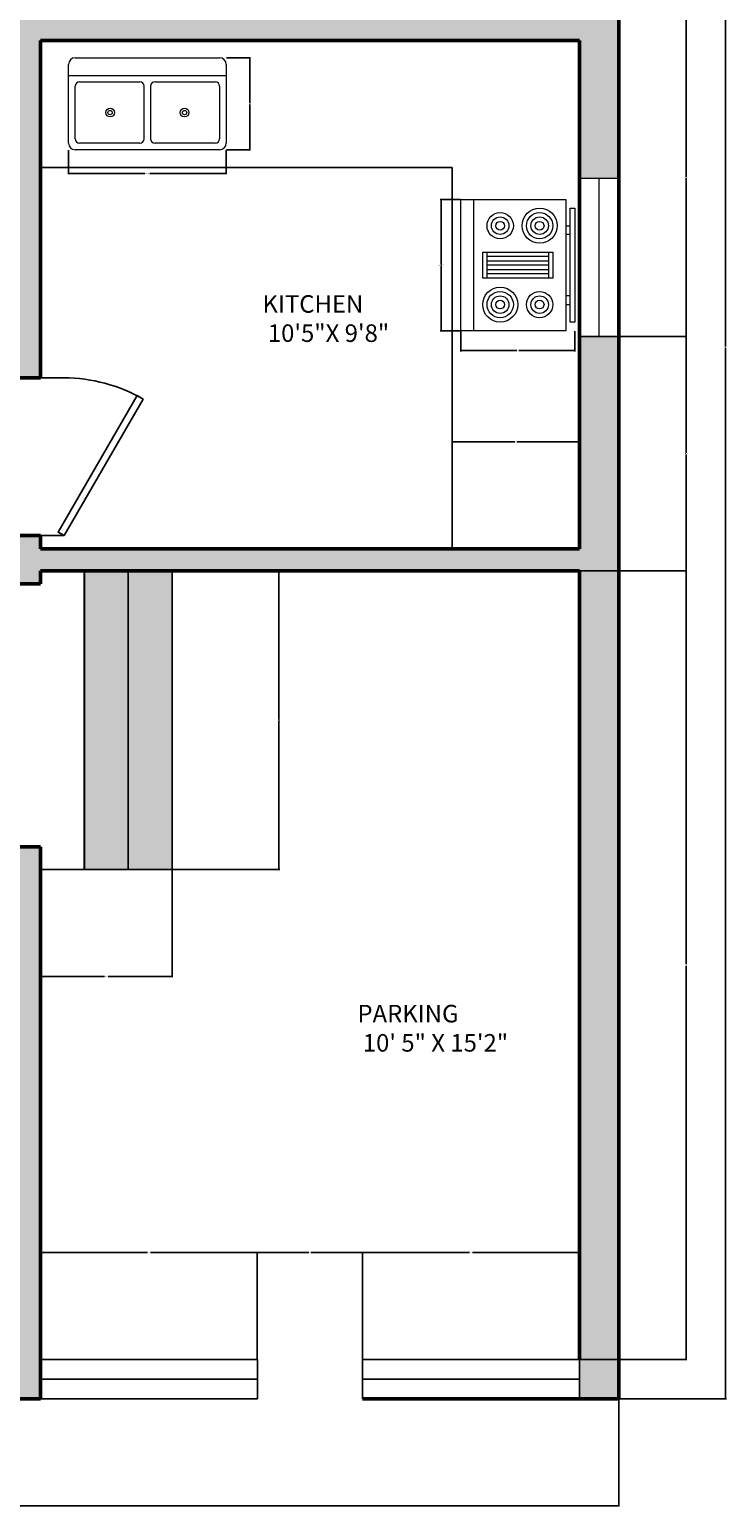
# Model space of a CAD drawing. Units: inches. Extents: x -23 to 411, y -22 to 507.
# Tile 3 of 5: x 252 to 411, y -22 to 315. Entities that reach past the tile are written whole.
import ezdxf

# ---------------------------------------------------------------- set-up
doc = ezdxf.new("R2010")
doc.units = ezdxf.units.IN
doc.header["$MEASUREMENT"] = 0
for name, color, linetype, lineweight in [('A-ANNO-DIMS', 2, 'Continuous', 18), ('A-AREA-IDEN', 7, 'Continuous', 25), ('A-EQPM', 181, 'Continuous', 18), ('A-FLOR-CASE', 181, 'Continuous', 25), ('A-FLOR-FIXT', 90, 'Continuous', 18), ('A-FLOR-STRS', 7, 'Continuous', 25), ('A-WALL', 7, 'Continuous', 50), ('doors', 40, 'Continuous', 25), ('window', 30, 'Continuous', 18)]:
    doc.layers.add(name, color=color, linetype=linetype, lineweight=lineweight)
doc.layers.add('A-FLOR-PATT', color=51, linetype='Continuous', lineweight=13, true_color=0xf8f6b0)
doc.layers.add('A-WALL-PATT', color=179, linetype='Continuous', lineweight=13, true_color=0x161b4b)
doc.styles.get("Standard").update_dxf_attribs({"font": 'arial.ttf'})
doc.dimstyles.get("Standard").update_dxf_attribs({"dimtxt": 0.18, "dimasz": 0.18, "dimexe": 0.18, "dimexo": 0.0625, "dimgap": 0.09, "dimtad": 0, "dimtih": 1, "dimtoh": 1, "dimdec": 4, "dimzin": 0, "dimdsep": 46, "dimtxsty": 'Standard', "dimcen": 0.09, "dimadec": 0, "dimazin": 0, "dimtfac": 1, "dimtdec": 4, "dimtofl": 0, "dimtmove": 0, "dimatfit": 3, "dimfxl": 1, "dimtolj": 1, "dimtzin": 0, "dimarcsym": 0})

# ---------------------------------------------------------------- blocks, each defined once
blk = doc.blocks.new('*U7')
for p, q in [((0, 0), (0, 6)), ((40, 0), (40, 6))]:
    blk.add_line(p, q)
blk.add_lwpolyline([(0, 0), (34.64, -20), (35.52, -18.48), (0.87, 1.52)], close=True)
blk.add_arc((0, 0), 40, 330, 0)
blk = doc.blocks.new('Range-Oven - 30 in top')
for p, q in [((0, -3), (30, -3)), ((12, -6), (18, -6)), ((13, -20), (13, -6)), ((14, -6), (14, -20)), ((15, -20), (15, -6)), ((16, -6), (16, -20)), ((17, -20), (17, -6)), ((18, -20), (12, -20)), ((6, -24), (6, -25)), ((8, -25), (8, -24)), ((22, -25), (22, -24)), ((24, -24), (24, -25))]:
    blk.add_line(p, q)
for points in [[(0, -24), (0, 0), (30, 0), (30, -24)], [(12, -21), (12, -5), (18, -5), (18, -21)], [(2, -26), (2, -25), (28, -25), (28, -26)]]:
    blk.add_lwpolyline(points, close=True)
for centre, radius in [((6, -9), 4), ((6, -9), 3), ((24, -9), 3), ((6, -9), 2), ((6, -9), 1), ((24, -9), 2), ((24, -9), 1), ((6, -18), 3), ((6, -18), 2), ((24, -18), 4), ((24, -18), 3), ((24, -18), 2), ((6, -18), 1), ((24, -18), 1)]:
    blk.add_circle(centre, radius)
blk = doc.blocks.new('Sink-double - 36 in top')
for p, q in [((-18, -4), (18, -4)), ((-0.75, -18.5), (-0.75, -6.5)), ((0.75, -6.5), (0.75, -18.5))]:
    blk.add_line(p, q)
for points in [[(-16.5, 0), (16.5, 0)], [(-18, -19.5), (-18, -1.5)], [(18, -1.5), (18, -19.5)], [(-16.5, -18.5), (-16.5, -6.5)], [(-15.5, -5.5), (-1.75, -5.5)], [(1.75, -5.5), (15.5, -5.5)], [(16.5, -6.5), (16.5, -18.5)], [(-1.75, -19.5), (-15.5, -19.5)], [(15.5, -19.5), (1.75, -19.5)], [(16.5, -21), (-16.5, -21)]]:
    blk.add_lwpolyline(points)
for centre, radius in [((-8.5, -12.5), 1), ((-8.5, -12.5), 0.5), ((8.5, -12.5), 1), ((8.5, -12.5), 0.5)]:
    blk.add_circle(centre, radius)
for centre, radius, start, end in [((-16.5, -1.5), 1.5, 90, 180), ((16.5, -1.5), 1.5, 0, 90), ((-15.5, -6.5), 1, 90, 180), ((-1.75, -6.5), 1, 0, 90), ((1.75, -6.5), 1, 90, 180), ((15.5, -6.5), 1, 0, 90), ((-16.5, -19.5), 1.5, 180, 270), ((-15.5, -18.5), 1, 180, 270), ((-1.75, -18.5), 1, 270, 0), ((1.75, -18.5), 1, 180, 270), ((15.5, -18.5), 1, 270, 0), ((16.5, -19.5), 1.5, 270, 0)]:
    blk.add_arc(centre, radius, start, end)
blk = doc.blocks.new('WIN-36IN')
for p, q in [((9, 36), (0, 36)), ((0, 36), (0, 0)), ((4.5, 0), (4.5, 36)), ((9, 0), (9, 36)), ((0, 0), (9, 0)), ((0, 0), (4.5, 0))]:
    blk.add_line(p, q)
blk = doc.blocks.new('*D22')
at = {"layer": 'A-ANNO-DIMS', "color": 0, "lineweight": -2, "transparency": 16777216}
for p, q in [((350.04, 276.62), (345.43, 276.62)), ((345.61, 276.44), (345.61, 261.81)), ((345.61, 246.8), (345.61, 261.44)), ((350.04, 246.62), (345.43, 246.62))]:
    blk.add_line(p, q, dxfattribs=at)
at = {"layer": 'A-ANNO-DIMS', "color": 0, "transparency": 16777216}
for points in [[(345.58, 276.44), (345.64, 276.44), (345.61, 276.62)], [(345.58, 246.8), (345.64, 246.8), (345.61, 246.62)]]:
    blk.add_solid(points, dxfattribs=at)
at = {"layer": 'Defpoints', "color": 0, "transparency": 16777216}
for p in [(345.61, 276.62), (350.11, 276.62), (350.11, 246.62)]:
    blk.add_point(p, dxfattribs=at)
at = {"layer": 'A-ANNO-DIMS', "color": 0, "transparency": 16777216, "insert": (345.61, 261.62), "char_height": 0.18, "attachment_point": 5}
blk.add_mtext('\\A1;RANGE 30', dxfattribs=at)
blk = doc.blocks.new('*D23')
at = {"layer": 'A-ANNO-DIMS', "color": 0, "lineweight": -2, "transparency": 16777216}
for p, q in [((350.11, 246.56), (350.11, 241.94)), ((376.11, 246.56), (376.11, 241.94)), ((350.29, 242.12), (362.89, 242.12)), ((375.93, 242.12), (363.33, 242.12))]:
    blk.add_line(p, q, dxfattribs=at)
at = {"layer": 'A-ANNO-DIMS', "color": 0, "transparency": 16777216}
for points in [[(350.29, 242.15), (350.29, 242.09), (350.11, 242.12)], [(375.93, 242.15), (375.93, 242.09), (376.11, 242.12)]]:
    blk.add_solid(points, dxfattribs=at)
at = {"layer": 'Defpoints', "color": 0, "transparency": 16777216}
for p in [(350.11, 246.62), (376.11, 246.62), (350.11, 242.12)]:
    blk.add_point(p, dxfattribs=at)
at = {"layer": 'A-ANNO-DIMS', "color": 0, "transparency": 16777216, "insert": (363.11, 242.12), "char_height": 0.18, "attachment_point": 5}
blk.add_mtext('\\A1;26', dxfattribs=at)
blk = doc.blocks.new('*D24')
at = {"layer": 'A-ANNO-DIMS', "color": 0, "lineweight": -2, "transparency": 16777216}
for p, q in [((260.57, 287.88), (260.57, 282.37)), ((296.57, 287.88), (296.57, 282.37)), ((260.75, 282.55), (278.02, 282.55)), ((296.39, 282.55), (279.12, 282.55))]:
    blk.add_line(p, q, dxfattribs=at)
at = {"layer": 'A-ANNO-DIMS', "color": 0, "transparency": 16777216}
for points in [[(260.75, 282.58), (260.75, 282.52), (260.57, 282.55)], [(296.39, 282.58), (296.39, 282.52), (296.57, 282.55)]]:
    blk.add_solid(points, dxfattribs=at)
at = {"layer": 'Defpoints', "color": 0, "transparency": 16777216}
for p in [(260.57, 287.95), (296.57, 287.95), (296.57, 282.55)]:
    blk.add_point(p, dxfattribs=at)
at = {"layer": 'A-ANNO-DIMS', "color": 0, "transparency": 16777216, "insert": (278.57, 282.55), "char_height": 0.18, "attachment_point": 5}
blk.add_mtext('\\A1;SINK 36', dxfattribs=at)
blk = doc.blocks.new('*D25')
at = {"layer": 'A-ANNO-DIMS', "color": 0, "lineweight": -2, "transparency": 16777216}
for p, q in [((296.63, 308.95), (302.15, 308.95)), ((301.97, 308.77), (301.97, 298.63)), ((301.97, 288.13), (301.97, 298.26)), ((296.63, 287.95), (302.15, 287.95))]:
    blk.add_line(p, q, dxfattribs=at)
at = {"layer": 'A-ANNO-DIMS', "color": 0, "transparency": 16777216}
for points in [[(301.94, 308.77), (302, 308.77), (301.97, 308.95)], [(301.94, 288.13), (302, 288.13), (301.97, 287.95)]]:
    blk.add_solid(points, dxfattribs=at)
at = {"layer": 'Defpoints', "color": 0, "transparency": 16777216}
for p in [(296.57, 308.95), (301.97, 308.95), (296.57, 287.95)]:
    blk.add_point(p, dxfattribs=at)
at = {"layer": 'A-ANNO-DIMS', "color": 0, "transparency": 16777216, "insert": (301.97, 298.45), "char_height": 0.18, "attachment_point": 5}
blk.add_mtext('\\A1;21', dxfattribs=at)
blk = doc.blocks.new('*D28')
at = {"layer": 'A-ANNO-DIMS', "color": 0, "lineweight": -2, "transparency": 16777216}
for p, q in [((2.17, 2.83), (2.17, -21.66)), ((386.17, 2.83), (386.17, -21.66)), ((2.35, -21.48), (193.89, -21.48)), ((385.99, -21.48), (194.46, -21.48))]:
    blk.add_line(p, q, dxfattribs=at)
at = {"layer": 'A-ANNO-DIMS', "color": 0, "transparency": 16777216}
for points in [[(2.35, -21.45), (2.35, -21.51), (2.17, -21.48)], [(385.99, -21.45), (385.99, -21.51), (386.17, -21.48)]]:
    blk.add_solid(points, dxfattribs=at)
at = {"layer": 'Defpoints', "color": 0, "transparency": 16777216}
for p in [(2.17, 2.9), (386.17, 2.9), (386.17, -21.48)]:
    blk.add_point(p, dxfattribs=at)
at = {"layer": 'A-ANNO-DIMS', "color": 0, "transparency": 16777216, "insert": (194.17, -21.48), "char_height": 0.18, "attachment_point": 5}
blk.add_mtext('\\A1;384', dxfattribs=at)
blk = doc.blocks.new('*D29')
at = {"layer": 'A-ANNO-DIMS', "color": 0, "lineweight": -2, "transparency": 16777216}
for p, q in [((386.24, 482.9), (410.73, 482.9)), ((410.55, 482.72), (410.55, 243.08)), ((410.55, 3.08), (410.55, 242.72)), ((386.24, 2.9), (410.73, 2.9))]:
    blk.add_line(p, q, dxfattribs=at)
at = {"layer": 'A-ANNO-DIMS', "color": 0, "transparency": 16777216}
for points in [[(410.52, 482.72), (410.58, 482.72), (410.55, 482.9)], [(410.52, 3.08), (410.58, 3.08), (410.55, 2.9)]]:
    blk.add_solid(points, dxfattribs=at)
at = {"layer": 'Defpoints', "color": 0, "transparency": 16777216}
for p in [(386.17, 482.9), (386.17, 2.9), (410.55, 2.9)]:
    blk.add_point(p, dxfattribs=at)
at = {"layer": 'A-ANNO-DIMS', "color": 0, "transparency": 16777216, "insert": (410.55, 242.9), "char_height": 0.18, "attachment_point": 5}
blk.add_mtext('\\A1;480', dxfattribs=at)
blk = doc.blocks.new('*D53')
at = {"layer": 'A-ANNO-DIMS', "color": 0, "lineweight": -2, "transparency": 16777216}
for p, q in [((377.24, 191.9), (401.73, 191.9)), ((401.55, 191.72), (401.55, 102.08)), ((401.55, 12.08), (401.55, 101.72)), ((377.24, 11.9), (401.73, 11.9))]:
    blk.add_line(p, q, dxfattribs=at)
at = {"layer": 'A-ANNO-DIMS', "color": 0, "transparency": 16777216}
for points in [[(401.52, 191.72), (401.58, 191.72), (401.55, 191.9)], [(401.52, 12.08), (401.58, 12.08), (401.55, 11.9)]]:
    blk.add_solid(points, dxfattribs=at)
at = {"layer": 'Defpoints', "color": 0, "transparency": 16777216}
for p in [(377.17, 191.9), (377.17, 11.9), (401.55, 11.9)]:
    blk.add_point(p, dxfattribs=at)
at = {"layer": 'A-ANNO-DIMS', "color": 0, "transparency": 16777216, "insert": (401.55, 101.9), "char_height": 0.18, "attachment_point": 5}
blk.add_mtext('\\A1;180', dxfattribs=at)
blk = doc.blocks.new('*D54')
at = {"layer": 'A-ANNO-DIMS', "color": 0, "lineweight": -2, "transparency": 16777216}
for p, q in [((377.24, 245.37), (401.73, 245.37)), ((401.55, 245.19), (401.55, 218.82)), ((401.55, 192.08), (401.55, 218.45)), ((377.24, 191.9), (401.73, 191.9))]:
    blk.add_line(p, q, dxfattribs=at)
at = {"layer": 'A-ANNO-DIMS', "color": 0, "transparency": 16777216}
for points in [[(401.52, 245.19), (401.58, 245.19), (401.55, 245.37)], [(401.52, 192.08), (401.58, 192.08), (401.55, 191.9)]]:
    blk.add_solid(points, dxfattribs=at)
at = {"layer": 'Defpoints', "color": 0, "transparency": 16777216}
for p in [(377.17, 245.37), (377.17, 191.9), (401.55, 191.9)]:
    blk.add_point(p, dxfattribs=at)
at = {"layer": 'A-ANNO-DIMS', "color": 0, "transparency": 16777216, "insert": (401.55, 218.64), "char_height": 0.18, "attachment_point": 5}
blk.add_mtext('\\A1;53.48', dxfattribs=at)
blk = doc.blocks.new('*D55')
at = {"layer": 'A-ANNO-DIMS', "color": 0, "lineweight": -2, "transparency": 16777216}
for p, q in [((377.24, 317.9), (401.73, 317.9)), ((401.55, 317.72), (401.55, 281.82)), ((401.55, 245.55), (401.55, 281.45)), ((377.24, 245.37), (401.73, 245.37))]:
    blk.add_line(p, q, dxfattribs=at)
at = {"layer": 'A-ANNO-DIMS', "color": 0, "transparency": 16777216}
for points in [[(401.52, 317.72), (401.58, 317.72), (401.55, 317.9)], [(401.52, 245.55), (401.58, 245.55), (401.55, 245.37)]]:
    blk.add_solid(points, dxfattribs=at)
at = {"layer": 'Defpoints', "color": 0, "transparency": 16777216}
for p in [(377.17, 317.9), (377.17, 245.37), (401.55, 245.37)]:
    blk.add_point(p, dxfattribs=at)
at = {"layer": 'A-ANNO-DIMS', "color": 0, "transparency": 16777216, "insert": (401.55, 281.64), "char_height": 0.18, "attachment_point": 5}
blk.add_mtext('\\A1;72.52', dxfattribs=at)
blk = doc.blocks.new('*D60')
at = {"layer": 'A-ANNO-DIMS', "color": 0, "lineweight": -2, "transparency": 16777216}
for p, q in [((254.17, 11.96), (254.17, 36.45)), ((254.35, 36.27), (278.6, 36.27)), ((303.49, 36.27), (279.25, 36.27)), ((303.67, 11.96), (303.67, 36.45))]:
    blk.add_line(p, q, dxfattribs=at)
at = {"layer": 'A-ANNO-DIMS', "color": 0, "transparency": 16777216}
for points in [[(254.35, 36.3), (254.35, 36.24), (254.17, 36.27)], [(303.49, 36.3), (303.49, 36.24), (303.67, 36.27)]]:
    blk.add_solid(points, dxfattribs=at)
at = {"layer": 'Defpoints', "color": 0, "transparency": 16777216}
for p in [(303.67, 36.27), (254.17, 11.9), (303.67, 11.9)]:
    blk.add_point(p, dxfattribs=at)
at = {"layer": 'A-ANNO-DIMS', "color": 0, "transparency": 16777216, "insert": (278.92, 36.27), "char_height": 0.18, "attachment_point": 5}
blk.add_mtext('\\A1;49.5', dxfattribs=at)
blk = doc.blocks.new('*D61')
at = {"layer": 'A-ANNO-DIMS', "color": 0, "lineweight": -2, "transparency": 16777216}
for p, q in [((303.67, 11.96), (303.67, 36.45)), ((303.85, 36.27), (315.45, 36.27)), ((327.49, 36.27), (315.89, 36.27)), ((327.67, 11.96), (327.67, 36.45))]:
    blk.add_line(p, q, dxfattribs=at)
at = {"layer": 'A-ANNO-DIMS', "color": 0, "transparency": 16777216}
for points in [[(303.85, 36.3), (303.85, 36.24), (303.67, 36.27)], [(327.49, 36.3), (327.49, 36.24), (327.67, 36.27)]]:
    blk.add_solid(points, dxfattribs=at)
at = {"layer": 'Defpoints', "color": 0, "transparency": 16777216}
for p in [(327.67, 36.27), (303.67, 11.9), (327.67, 11.9)]:
    blk.add_point(p, dxfattribs=at)
at = {"layer": 'A-ANNO-DIMS', "color": 0, "transparency": 16777216, "insert": (315.67, 36.27), "char_height": 0.18, "attachment_point": 5}
blk.add_mtext('\\A1;24', dxfattribs=at)
blk = doc.blocks.new('*D62')
at = {"layer": 'A-ANNO-DIMS', "color": 0, "lineweight": -2, "transparency": 16777216}
for p, q in [((327.67, 11.96), (327.67, 36.45)), ((327.85, 36.27), (352.1, 36.27)), ((376.99, 36.27), (352.75, 36.27)), ((377.17, 11.96), (377.17, 36.45))]:
    blk.add_line(p, q, dxfattribs=at)
at = {"layer": 'A-ANNO-DIMS', "color": 0, "transparency": 16777216}
for points in [[(327.85, 36.3), (327.85, 36.24), (327.67, 36.27)], [(376.99, 36.3), (376.99, 36.24), (377.17, 36.27)]]:
    blk.add_solid(points, dxfattribs=at)
at = {"layer": 'Defpoints', "color": 0, "transparency": 16777216}
for p in [(377.17, 36.27), (327.67, 11.9), (377.17, 11.9)]:
    blk.add_point(p, dxfattribs=at)
at = {"layer": 'A-ANNO-DIMS', "color": 0, "transparency": 16777216, "insert": (352.42, 36.27), "char_height": 0.18, "attachment_point": 5}
blk.add_mtext('\\A1;49.5', dxfattribs=at)
blk = doc.blocks.new('*D63')
at = {"layer": 'A-ANNO-DIMS', "color": 0, "lineweight": -2, "transparency": 16777216}
for p, q in [((348.17, 196.96), (348.17, 221.45)), ((348.35, 221.27), (362.45, 221.27)), ((376.99, 221.27), (362.9, 221.27)), ((377.17, 196.96), (377.17, 221.45))]:
    blk.add_line(p, q, dxfattribs=at)
at = {"layer": 'A-ANNO-DIMS', "color": 0, "transparency": 16777216}
for points in [[(348.35, 221.3), (348.35, 221.24), (348.17, 221.27)], [(376.99, 221.3), (376.99, 221.24), (377.17, 221.27)]]:
    blk.add_solid(points, dxfattribs=at)
at = {"layer": 'Defpoints', "color": 0, "transparency": 16777216}
for p in [(377.17, 221.27), (348.17, 196.9), (377.17, 196.9)]:
    blk.add_point(p, dxfattribs=at)
at = {"layer": 'A-ANNO-DIMS', "color": 0, "transparency": 16777216, "insert": (362.67, 221.27), "char_height": 0.18, "attachment_point": 5}
blk.add_mtext('\\A1;29', dxfattribs=at)
blk = doc.blocks.new('*D64')
at = {"layer": 'A-ANNO-DIMS', "color": 0, "lineweight": -2, "transparency": 16777216}
for p, q in [((254.17, 123.61), (254.17, 99.11)), ((284.21, 123.61), (284.21, 99.11)), ((254.35, 99.29), (268.8, 99.29)), ((284.03, 99.29), (269.59, 99.29))]:
    blk.add_line(p, q, dxfattribs=at)
at = {"layer": 'A-ANNO-DIMS', "color": 0, "transparency": 16777216}
for points in [[(254.35, 99.32), (254.35, 99.26), (254.17, 99.29)], [(284.03, 99.32), (284.03, 99.26), (284.21, 99.29)]]:
    blk.add_solid(points, dxfattribs=at)
at = {"layer": 'Defpoints', "color": 0, "transparency": 16777216}
for p in [(254.17, 123.67), (284.21, 123.67), (254.17, 99.29)]:
    blk.add_point(p, dxfattribs=at)
at = {"layer": 'A-ANNO-DIMS', "color": 0, "transparency": 16777216, "insert": (269.19, 99.29), "char_height": 0.18, "attachment_point": 5}
blk.add_mtext('\\A1;30.04', dxfattribs=at)
blk = doc.blocks.new('*D65')
at = {"layer": 'A-ANNO-DIMS', "color": 0, "lineweight": -2, "transparency": 16777216}
for p, q in [((284.27, 191.9), (308.77, 191.9)), ((308.59, 191.72), (308.59, 157.97)), ((308.59, 123.85), (308.59, 157.6)), ((284.27, 123.67), (308.77, 123.67))]:
    blk.add_line(p, q, dxfattribs=at)
at = {"layer": 'A-ANNO-DIMS', "color": 0, "transparency": 16777216}
for points in [[(308.56, 191.72), (308.62, 191.72), (308.59, 191.9)], [(308.56, 123.85), (308.62, 123.85), (308.59, 123.67)]]:
    blk.add_solid(points, dxfattribs=at)
at = {"layer": 'Defpoints', "color": 0, "transparency": 16777216}
for p in [(284.21, 191.9), (284.21, 123.67), (308.59, 123.67)]:
    blk.add_point(p, dxfattribs=at)
at = {"layer": 'A-ANNO-DIMS', "color": 0, "transparency": 16777216, "insert": (308.59, 157.78), "char_height": 0.18, "attachment_point": 5}
blk.add_mtext('\\A1;68.23', dxfattribs=at)

msp = doc.modelspace()

# ---------------------------------------------------------------- hatches: boundary and pattern name
at = {"layer": 'A-FLOR-PATT'}
h = msp.add_hatch(color=256, dxfattribs=at)
h.dxf.hatch_style = 1
h.paths.add_polyline_path([(284.2118, 191.8972), (274.2118, 191.8972), (274.2118, 123.6717), (284.2118, 123.6717)])
h.paths.add_polyline_path([(274.2118, 191.8972), (264.2118, 191.8972), (264.2118, 123.6717), (274.2118, 123.6717)])
at = {"layer": 'A-WALL-PATT'}
h = msp.add_hatch(color=256, dxfattribs=at)
h.dxf.hatch_style = 1
h.paths.add_polyline_path([(37.3453, 482.8972), (2.1746, 482.8972), (2.1746, 414.9823), (11.1746, 414.9823), (11.1746, 473.8972), (37.3453, 473.8972)])
h.paths.add_polyline_path([(149.2817, 482.8972), (73.3453, 482.8972), (73.3453, 473.8972), (131.1746, 473.8972), (131.1746, 356.8972), (136.1746, 356.8972), (136.1746, 372.8972), (139.1746, 372.8972), (139.1746, 377.8972), (136.1746, 377.8972), (136.1746, 473.8972), (149.2817, 473.8972)])
h.paths.add_polyline_path([(209.1361, 482.8972), (173.2817, 482.8972), (173.2817, 473.8972), (190.1746, 473.8972), (190.1746, 377.8972), (168.1746, 377.8972), (168.1746, 372.8972), (249.1746, 372.8972), (249.1746, 356.8972), (254.1746, 356.8972), (254.1746, 380.8972), (249.1746, 380.8972), (249.1746, 377.8972), (195.1746, 377.8972), (195.1746, 473.8972), (209.1361, 473.8972)])
h.paths.add_polyline_path([(309.9724, 482.8972), (233.1361, 482.8972), (233.1361, 473.8972), (249.1746, 473.8972), (249.1746, 409.8972), (254.1746, 409.8972), (254.1746, 473.8972), (309.9724, 473.8972)])
h.paths.add_polyline_path([(386.1746, 482.8972), (345.9724, 482.8972), (345.9724, 473.8972), (377.1746, 473.8972), (377.1746, 445.6454), (386.1746, 445.6454)])
h.paths.add_polyline_path([(386.1746, 409.6454), (377.1746, 409.6454), (377.1746, 317.8972), (254.1746, 317.8972), (254.1746, 320.8972), (249.1746, 320.8972), (249.1746, 317.8972), (249.1746, 235.8972), (254.1746, 235.8972), (254.1746, 312.8972), (377.1746, 312.8972), (377.1746, 281.3732), (386.1746, 281.3732)])
h.paths.add_polyline_path([(386.1746, 245.3732), (377.1746, 245.3732), (377.1746, 196.8972), (254.1746, 196.8972), (254.1746, 199.8972), (249.1746, 199.8972), (249.1746, 196.8972), (249.1746, 188.8972), (254.1746, 188.8972), (254.1746, 191.8972), (264.1746, 191.8972), (377.1746, 191.8972), (377.1746, 11.8972), (377.1746, 2.8972), (386.1746, 2.8972)])
h.paths.add_polyline_path([(254.1746, 128.8972), (249.1746, 128.8972), (249.1746, 11.8972), (206.9157, 11.8972), (206.9157, 2.8972), (254.1746, 2.8972)])
h.paths.add_polyline_path([(170.9157, 11.8972), (86.2116, 11.8972), (86.2116, 2.8972), (170.9157, 2.8972)])
h.paths.add_polyline_path([(136.1746, 114.8972), (131.1746, 114.8972), (131.1746, 11.8972), (136.1746, 11.8972)])
h.paths.add_polyline_path([(50.2116, 11.8972), (11.1746, 11.8972), (11.1746, 90.1201), (2.1746, 90.1201), (2.1746, 2.8972), (50.2116, 2.8972)])
h.paths.add_polyline_path([(11.1746, 176.2548), (2.1746, 176.2548), (2.1746, 126.1201), (11.1746, 126.1201)])
h.paths.add_polyline_path([(136.1746, 158.8972), (11.1746, 158.8972), (11.1746, 153.8972), (131.1746, 153.8972), (131.1746, 150.8972), (136.1746, 150.8972)])
h.paths.add_polyline_path([(11.1746, 269.5052), (2.1746, 269.5052), (2.1746, 212.2548), (11.1746, 212.2548)])
h.paths.add_polyline_path([(11.1746, 378.9823), (2.1746, 378.9823), (2.1746, 305.5052), (11.1746, 305.5052), (11.1746, 312.8972), (136.1746, 312.8972), (136.1746, 320.8972), (131.1746, 320.8972), (131.1746, 317.8972), (11.1746, 317.8972)])

# ---------------------------------------------------------------- linework, layer by layer
at = {"layer": 'A-FLOR-CASE'}
for p, q in [((254.1746, 312.8972), (254.1746, 283.8972)), ((377.1746, 312.8972), (348.1746, 312.8972)), ((254.1746, 283.8972), (348.1746, 283.8972)), ((348.1746, 283.8972), (348.1746, 196.8972))]:
    msp.add_line(p, q, dxfattribs=at)
at = {"layer": 'A-FLOR-STRS'}
for p, q in [((254.1746, 191.8972), (264.1746, 191.8972)), ((264.1746, 191.8972), (264.1746, 123.6717)), ((264.2118, 191.8972), (264.2118, 123.6717)), ((274.2118, 191.8972), (274.2118, 123.6717)), ((284.2118, 191.8972), (284.2118, 123.6717)), ((284.2118, 123.6717), (254.1746, 123.6717))]:
    msp.add_line(p, q, dxfattribs=at)
at = {"layer": 'A-WALL'}
for p, q in [((254.1746, 312.8972), (377.1746, 312.8972)), ((254.1746, 235.8972), (254.1746, 312.8972)), ((377.1746, 312.8972), (377.1746, 196.8972)), ((254.1746, 235.8972), (249.1746, 235.8972)), ((249.1746, 199.8972), (254.1746, 199.8972)), ((254.1746, 196.8972), (254.1746, 199.8972)), ((254.1746, 196.8972), (377.1746, 196.8972)), ((249.1746, 188.8972), (254.1746, 188.8972)), ((254.1746, 191.8972), (377.1746, 191.8972)), ((254.1746, 188.8972), (254.1746, 191.8972)), ((377.1746, 191.8972), (377.1746, 11.8972)), ((249.1746, 128.8972), (254.1746, 128.8972)), ((254.1746, 2.8972), (254.1746, 128.8972))]:
    msp.add_line(p, q, dxfattribs=at)
for points in [[(254.1746, 2.8972), (2.1746, 2.8972), (2.1746, 482.8972), (386.1746, 482.8972), (386.1746, 2.8972), (377.1746, 2.8972)], [(386.1746, 2.8972), (327.6746, 2.8972)]]:
    msp.add_lwpolyline(points, dxfattribs=at)
at = {"layer": 'doors'}
for p, q in [((303.6746, 11.8972), (254.1746, 11.8972)), ((254.1746, 11.8972), (303.6746, 11.8972)), ((254.1746, 11.8972), (290.1746, 11.8972)), ((303.6746, 11.8972), (303.6746, 2.8972)), ((377.1746, 11.8972), (327.6746, 11.8972)), ((327.6746, 11.8972), (377.1746, 11.8972)), ((327.6746, 11.8972), (327.6746, 2.8972)), ((377.1746, 11.8972), (377.1746, 2.8972)), ((303.6746, 7.3972), (254.1746, 7.3972)), ((377.1746, 7.3972), (327.6746, 7.3972))]:
    msp.add_line(p, q, dxfattribs=at)
for points in [[(303.6746, 2.8972), (254.1746, 2.8972)], [(377.1746, 2.8972), (327.6746, 2.8972)]]:
    msp.add_lwpolyline(points, dxfattribs=at)

# ---------------------------------------------------------------- block references
at = {"layer": 'A-EQPM', "rotation": 89.99999999999999}
msp.add_blockref('Range-Oven - 30 in top', (350.107, 246.6244), dxfattribs=at)
at = {"layer": 'A-FLOR-FIXT'}
msp.add_blockref('Sink-double - 36 in top', (278.5682, 308.9451), dxfattribs=at)
at = {"layer": 'doors', "xscale": 0.9, "yscale": 0.9, "zscale": 0.9, "rotation": 90}
msp.add_blockref('*U7', (259.5746, 199.8972), dxfattribs=at)
at = {"layer": 'window'}
msp.add_blockref('WIN-36IN', (377.175, 245.373), dxfattribs=at)

# ---------------------------------------------------------------- texts
at = {"layer": 'A-AREA-IDEN', "char_height": 4, "attachment_point": 1}
for s, insert in [('KITCHEN\\P 10\'5"X 9\'8"', (304.8479, 254.7765)), ('PARKING\\P 10\' 5" X 15\'2"', (326.5211, 92.8123))]:
    msp.add_mtext_dynamic_manual_height_columns(s, width=61.991846, gutter_width=1, heights=[0], dxfattribs=dict(at, insert=insert))

# ---------------------------------------------------------------- dimensions: what is measured, and where the dimension line sits
at = {"layer": 'A-ANNO-DIMS'}
for base, p1, p2, angle, override, picture, middle in [((410.5521, 2.8972), (386.1746, 482.8972), (386.1746, 2.8972), 270, {"dimdec": 0, "dimlfac": 1, "dimrnd": 0, "dimzin": 0, "dimdsep": 46, "dimlunit": 2}, '*D29', (410.5521, 242.8972)), ((401.5521, 245.3732), (377.1746, 317.8972), (377.1746, 245.3732), 270, {"dimdec": 2, "dimlfac": 1, "dimrnd": 0, "dimzin": 0, "dimdsep": 46, "dimlunit": 2}, '*D55', (401.5521, 281.6352)), ((301.9682, 308.9451), (296.5682, 287.9451), (296.5682, 308.9451), 90, {"dimdec": 0, "dimlfac": 1, "dimrnd": 0, "dimzin": 0, "dimdsep": 46, "dimlunit": 2}, '*D25', (301.9682, 298.4451)), ((350.107, 242.1244), (376.107, 246.6244), (350.107, 246.6244), 180, {"dimdec": 0, "dimlfac": 1, "dimrnd": 0, "dimzin": 0, "dimdsep": 46, "dimlunit": 2}, '*D23', (363.107, 242.1244)), ((401.5521, 191.8972), (377.1746, 245.3732), (377.1746, 191.8972), 270, {"dimdec": 2, "dimlfac": 1, "dimrnd": 0, "dimzin": 0, "dimdsep": 46, "dimlunit": 2}, '*D54', (401.5521, 218.6352)), ((308.5893, 123.6717), (284.2118, 191.8972), (284.2118, 123.6717), 270, {"dimdec": 2, "dimlfac": 1, "dimrnd": 0, "dimzin": 0, "dimdsep": 46, "dimlunit": 2}, '*D65', (308.5893, 157.7844)), ((401.5521, 11.8972), (377.1746, 191.8972), (377.1746, 11.8972), 270, {"dimdec": 0, "dimlfac": 1, "dimrnd": 0, "dimzin": 0, "dimdsep": 46, "dimlunit": 2}, '*D53', (401.5521, 101.8972)), ((254.1746, 99.2942), (284.2118, 123.6717), (254.1746, 123.6717), 180, {"dimdec": 2, "dimlfac": 1, "dimrnd": 0, "dimzin": 0, "dimdsep": 46, "dimlunit": 2}, '*D64', (269.1932, 99.2942))]:
    dim = msp.add_linear_dim(base=base, p1=p1, p2=p2, angle=angle, dimstyle='Standard', override=override, dxfattribs=at)
    dim.commit()
    dim.dimension.update_dxf_attribs({"geometry": picture, "text_midpoint": middle})
dim = msp.add_linear_dim(base=(296.5682, 282.5451), p1=(260.5682, 287.9451), p2=(296.5682, 287.9451), text='SINK <>', dimstyle='Standard', override={"dimdec": 0, "dimlfac": 1, "dimrnd": 0, "dimzin": 0, "dimdsep": 46, "dimlunit": 2}, dxfattribs=at)
dim.commit()
dim.dimension.update_dxf_attribs({"geometry": '*D24', "text_midpoint": (278.5682, 282.5451)})
dim = msp.add_linear_dim(base=(345.607, 276.6244), p1=(350.107, 246.6244), p2=(350.107, 276.6244), angle=90, text='RANGE <>', dimstyle='Standard', override={"dimdec": 0, "dimlfac": 1, "dimrnd": 0, "dimzin": 0, "dimdsep": 46, "dimlunit": 2}, dxfattribs=at)
dim.commit()
dim.dimension.update_dxf_attribs({"geometry": '*D22', "text_midpoint": (345.607, 261.6244)})
for base, p1, p2, override, picture, middle in [((377.1746, 221.2747), (348.1746, 196.8972), (377.1746, 196.8972), {"dimdec": 0, "dimlfac": 1, "dimrnd": 0, "dimzin": 0, "dimdsep": 46, "dimlunit": 2}, '*D63', (362.6746, 221.2747)), ((303.6746, 36.2747), (254.1746, 11.8972), (303.6746, 11.8972), {"dimdec": 1, "dimlfac": 1, "dimrnd": 0, "dimzin": 0, "dimdsep": 46, "dimlunit": 2}, '*D60', (278.9246, 36.2747)), ((327.6746, 36.2747), (303.6746, 11.8972), (327.6746, 11.8972), {"dimdec": 0, "dimlfac": 1, "dimrnd": 0, "dimzin": 0, "dimdsep": 46, "dimlunit": 2}, '*D61', (315.6746, 36.2747)), ((377.1746, 36.2747), (327.6746, 11.8972), (377.1746, 11.8972), {"dimdec": 1, "dimlfac": 1, "dimrnd": 0, "dimzin": 0, "dimdsep": 46, "dimlunit": 2}, '*D62', (352.4246, 36.2747)), ((386.1746, -21.4803), (2.1746, 2.8972), (386.1746, 2.8972), {"dimdec": 0, "dimlfac": 1, "dimrnd": 0, "dimzin": 0, "dimdsep": 46, "dimlunit": 2}, '*D28', (194.1746, -21.4803))]:
    dim = msp.add_linear_dim(base=base, p1=p1, p2=p2, dimstyle='Standard', override=override, dxfattribs=at)
    dim.commit()
    dim.dimension.update_dxf_attribs({"geometry": picture, "text_midpoint": middle})

doc.saveas('drawing.dxf')
